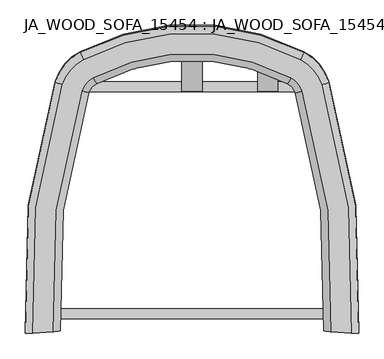
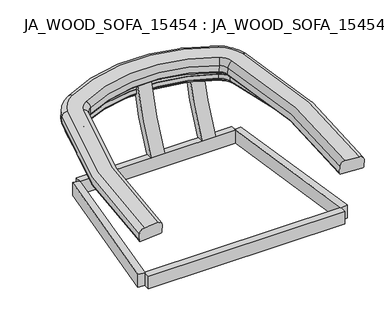
"""IFC4 building model written with IfcOpenShell, lengths in millimetres: furniture geometry, JA_WOOD_SOFA_15454 : JA_WOOD_SOFA_15454."""

from ifc_helpers import new_model, si_unit, point, frame, frame_2d, origin, place, context, project, spatial, polyline, circle_curve, ellipse_curve, trimmed, segment, composite_curve, outline, extrude, source, transform, mapped, element, save
from ifc_brep_helpers import plane_surface, cylinder_surface, revolved_surface, advanced_brep


def ja_wood_sofa_15454_ja_wood_sofa_15454_f522b914(model_context):
    return source(origin(), model_context, "Body", "SolidModel", [
        advanced_brep(
        [(-275.4813305, -35.2597244, 497.0679673), (-315.380229, -38.0910735, 496.8202564), (-330.3423159, -37.8454933, 481.7844443), (-330.3423159, -36.1023784, 461.8605503), (-325.3549536, -35.3126811, 456.9105407), (-265.5066059, -31.0656574, 457.2821072), (-260.5192436, -31.1475174, 462.2940445), (-260.5192436, -32.8906323, 482.2179385), (-256.5569192, 453.6794856, 539.8446054), (-218.4430808, 441.5874987, 538.7866936), (-196.0745351, 468.1438524, 541.1100735), (196.0745351, 468.1438524, 541.1100735), (218.4430808, 441.5874987, 538.7866936), (275.4813305, -35.2597244, 497.0679673), (315.380229, -38.0910735, 496.8202564), (256.5569192, 453.6794856, 539.8446054), (214.6467039, 503.4360732, 544.1977427), (-214.6467039, 503.4360732, 544.1977427), (-270.8496086, 461.2644317, 505.3745079), (-270.8496086, 459.5213169, 525.2984018), (-208.9146212, 442.0507317, 498.6744277), (-266.0853788, 460.1887121, 500.2612954), (-219.2897461, 515.7453581, 505.1218721), (219.2897461, 515.7453581, 505.1218721), (266.0853788, 460.1887121, 500.2612954), (325.3549536, -35.3126811, 456.9105407), (265.5066059, -31.0656574, 457.2821072), (208.9146212, 442.0507317, 498.6744277), (191.4314929, 462.8070269, 500.4903683), (-191.4314929, 462.8070269, 500.4903683), (-204.1503914, 438.3603397, 523.4470562), (-204.1503914, 440.1034546, 503.5231622), (-221.6112672, 519.7211069, 510.4888042), (-221.6112672, 517.9779921, 530.4126982), (-189.1099718, 456.2166058, 525.0092771), (-189.1099718, 457.9597206, 505.0853831), (221.6112672, 519.7211069, 510.4888042), (221.6112672, 517.9779921, 530.4126982), (189.1099718, 456.2166058, 525.0092771), (189.1099718, 457.9597206, 505.0853831), (270.8496086, 461.2644317, 505.3745079), (270.8496086, 459.5213169, 525.2984018), (204.1503914, 438.3603397, 523.4470562), (204.1503914, 440.1034546, 503.5231622), (260.5192436, -32.8906323, 482.2179385), (260.5192436, -31.1475174, 462.2940445), (330.3423159, -36.1023784, 461.8605503), (330.3423159, -37.8454933, 481.7844443)],
        [
            (0, 1),
            (1, 2, circle_curve(frame((-315.380229, -36.7837374, 481.8773359), z_axis=(0.07105411082948589, -0.9936767785792983, -0.08693545333464162), x_axis=(-0.9974724624440673, -0.07078372848595715, -0.006192773804617793)), 15.0)),
            (2, 3),
            (3, 4, circle_curve(frame((-325.3549536, -35.7484598, 461.8915142), z_axis=(0.07105411082948589, -0.9936767785792983, -0.08693545333464162), x_axis=(-0.9974724624440673, -0.07078372848595715, -0.006192773804617793)), 5.0)),
            (4, 5),
            (5, 6, circle_curve(frame((-265.5066059, -31.5014361, 462.2630806), z_axis=(0.07105411082948589, -0.9936767785792983, -0.08693545333464162), x_axis=(-0.9974724624440673, -0.07078372848595715, -0.006192773804617793)), 5.0)),
            (6, 7),
            (7, 0, circle_curve(frame((-275.4813305, -33.9523882, 482.1250469), z_axis=(0.07105411082948589, -0.9936767785792983, -0.08693545333464162), x_axis=(-0.9974724624440673, -0.07078372848595715, -0.006192773804617793)), 15.0)),
            (8, 1, circle_curve(frame((999.4131606, 55.2107286, 504.9831064), z_axis=(0.0, -0.08715574274765152, 0.9961946980917462), x_axis=(-0.9974724624440673, -0.07078372848595717, -0.006192773804617792)), 1318.125)),
            (0, 9, circle_curve(frame((999.4131606, 55.2107286, 504.9831064), z_axis=(0.0, 0.08715574274765152, -0.9961946980917462), x_axis=(-0.9974724624440673, -0.07078372848595717, -0.006192773804617792)), 1278.125)),
            (9, 10, circle_curve(frame((-174.8157372, 427.7462984, 537.5757455), z_axis=(0.0, 0.08715574274765152, -0.9961946980917462), x_axis=(-0.9528459590255555, 0.3022996734028965, 0.026447794410340692)), 45.7863553)),
            (10, 11, circle_curve(frame((0.0, 95.5483916, 508.5121946), z_axis=(0.0, 0.08715574274765152, -0.9961946980917462), x_axis=(-0.4643042190951026, 0.8823055189929315, 0.0771917306782324)), 422.2975521)),
            (11, 12, circle_curve(frame((174.8157372, 427.7462984, 537.5757455), z_axis=(0.0, 0.08715574274765152, -0.9961946980917462), x_axis=(0.46430421909505437, 0.8823055189929567, 0.0771917306782346)), 45.7863553)),
            (12, 13, circle_curve(frame((-999.4131606, 55.2107286, 504.9831064), z_axis=(0.0, 0.08715574274765152, -0.9961946980917462), x_axis=(0.9528459590255144, 0.3022996734030248, 0.026447794410351923)), 1278.125)),
            (13, 14),
            (14, 15, circle_curve(frame((-999.4131606, 55.2107286, 504.9831064), z_axis=(0.0, -0.08715574274765152, 0.9961946980917462), x_axis=(0.9528459590255144, 0.3022996734030248, 0.026447794410351923)), 1318.125)),
            (15, 16, circle_curve(frame((174.8157372, 427.7462984, 537.5757455), z_axis=(0.0, -0.08715574274765152, 0.9961946980917462), x_axis=(0.46430421909505437, 0.8823055189929567, 0.0771917306782346)), 85.7863553)),
            (16, 17, circle_curve(frame((0.0, 95.5483916, 508.5121946), z_axis=(0.0, -0.08715574274765152, 0.9961946980917462), x_axis=(-0.4643042190951026, 0.8823055189929315, 0.0771917306782324)), 462.2975521)),
            (17, 8, circle_curve(frame((-174.8157372, 427.7462984, 537.5757455), z_axis=(0.0, -0.08715574274765152, 0.9961946980917462), x_axis=(-0.9528459590255555, 0.3022996734028965, 0.026447794410340692)), 85.7863553)),
            (18, 3, circle_curve(frame((999.4131606, 58.2611796, 470.1162919), z_axis=(0.0, -0.08715574274765152, 0.9961946980917462), x_axis=(-0.9974724624440673, -0.07078372848595717, -0.006192773804617792)), 1333.125)),
            (2, 19, circle_curve(frame((999.4131606, 56.5180648, 490.0401859), z_axis=(0.0, 0.08715574274765152, -0.9961946980917462), x_axis=(-0.9974724624440673, -0.07078372848595717, -0.006192773804617792)), 1333.125)),
            (19, 18),
            (20, 5, circle_curve(frame((999.4131606, 58.6969583, 465.1353184), z_axis=(0.0, -0.08715574274765152, 0.9961946980917462), x_axis=(-0.9974724624440673, -0.07078372848595717, -0.006192773804617792)), 1268.125)),
            (4, 21, circle_curve(frame((999.4131606, 58.6969583, 465.1353184), z_axis=(0.0, 0.08715574274765152, -0.9961946980917462), x_axis=(-0.9974724624440673, -0.07078372848595717, -0.006192773804617792)), 1328.125)),
            (21, 22, circle_curve(frame((-174.8157372, 431.2325281, 497.7279576), z_axis=(0.0, 0.08715574274765152, -0.9961946980917462), x_axis=(-0.9528459590255555, 0.3022996734028965, 0.026447794410340692)), 95.7863553)),
            (22, 23, circle_curve(frame((0.0, 99.0346213, 468.6644067), z_axis=(0.0, 0.08715574274765152, -0.9961946980917462), x_axis=(-0.4643042190951026, 0.8823055189929315, 0.0771917306782324)), 472.2975521)),
            (23, 24, circle_curve(frame((174.8157372, 431.2325281, 497.7279576), z_axis=(0.0, 0.08715574274765152, -0.9961946980917462), x_axis=(0.46430421909505437, 0.8823055189929567, 0.0771917306782346)), 95.7863553)),
            (24, 25, circle_curve(frame((-999.4131606, 58.6969583, 465.1353184), z_axis=(0.0, 0.08715574274765152, -0.9961946980917462), x_axis=(0.9528459590255144, 0.3022996734030248, 0.026447794410351923)), 1328.125)),
            (25, 26),
            (26, 27, circle_curve(frame((-999.4131606, 58.6969583, 465.1353184), z_axis=(0.0, -0.08715574274765152, 0.9961946980917462), x_axis=(0.9528459590255144, 0.3022996734030248, 0.026447794410351923)), 1268.125)),
            (27, 28, circle_curve(frame((174.8157372, 431.2325281, 497.7279576), z_axis=(0.0, -0.08715574274765152, 0.9961946980917462), x_axis=(0.46430421909505437, 0.8823055189929567, 0.0771917306782346)), 35.7863553)),
            (28, 29, circle_curve(frame((0.0, 99.0346213, 468.6644067), z_axis=(0.0, -0.08715574274765152, 0.9961946980917462), x_axis=(-0.4643042190951026, 0.8823055189929315, 0.0771917306782324)), 412.2975521)),
            (29, 20, circle_curve(frame((-174.8157372, 431.2325281, 497.7279576), z_axis=(0.0, -0.08715574274765152, 0.9961946980917462), x_axis=(-0.9528459590255555, 0.3022996734028965, 0.026447794410340692)), 35.7863553)),
            (30, 7, circle_curve(frame((999.4131606, 56.5180648, 490.0401859), z_axis=(0.0, -0.08715574274765152, 0.9961946980917462), x_axis=(-0.9974724624440673, -0.07078372848595717, -0.006192773804617792)), 1263.125)),
            (6, 31, circle_curve(frame((999.4131606, 58.2611796, 470.1162919), z_axis=(0.0, 0.08715574274765152, -0.9961946980917462), x_axis=(-0.9974724624440673, -0.07078372848595717, -0.006192773804617792)), 1263.125)),
            (31, 30),
            (32, 18, circle_curve(frame((-174.8157372, 430.7967494, 502.708931), z_axis=(0.0, -0.08715574274765152, 0.9961946980917462), x_axis=(-0.9528459590255555, 0.3022996734028965, 0.026447794410340692)), 100.7863553)),
            (19, 33, circle_curve(frame((-174.8157372, 429.0536346, 522.632825), z_axis=(0.0, 0.08715574274765152, -0.9961946980917462), x_axis=(-0.9528459590255555, 0.3022996734028965, 0.026447794410340692)), 100.7863553)),
            (33, 32),
            (34, 30, circle_curve(frame((-174.8157372, 429.0536346, 522.632825), z_axis=(0.0, -0.08715574274765152, 0.9961946980917462), x_axis=(-0.9528459590255555, 0.3022996734028965, 0.026447794410340692)), 30.7863553)),
            (31, 35, circle_curve(frame((-174.8157372, 430.7967494, 502.708931), z_axis=(0.0, 0.08715574274765152, -0.9961946980917462), x_axis=(-0.9528459590255555, 0.3022996734028965, 0.026447794410340692)), 30.7863553)),
            (35, 34),
            (36, 32, circle_curve(frame((0.0, 98.5988426, 473.6453801), z_axis=(0.0, -0.08715574274765152, 0.9961946980917462), x_axis=(-0.4643042190951026, 0.8823055189929315, 0.0771917306782324)), 477.2975521)),
            (33, 37, circle_curve(frame((0.0, 96.8557277, 493.5692741), z_axis=(0.0, 0.08715574274765152, -0.9961946980917462), x_axis=(-0.4643042190951026, 0.8823055189929315, 0.0771917306782324)), 477.2975521)),
            (37, 36),
            (38, 34, circle_curve(frame((0.0, 96.8557277, 493.5692741), z_axis=(0.0, -0.08715574274765152, 0.9961946980917462), x_axis=(-0.4643042190951026, 0.8823055189929315, 0.0771917306782324)), 407.2975521)),
            (35, 39, circle_curve(frame((0.0, 98.5988426, 473.6453801), z_axis=(0.0, 0.08715574274765152, -0.9961946980917462), x_axis=(-0.4643042190951026, 0.8823055189929315, 0.0771917306782324)), 407.2975521)),
            (39, 38),
            (40, 36, circle_curve(frame((174.8157372, 430.7967494, 502.708931), z_axis=(0.0, -0.08715574274765152, 0.9961946980917462), x_axis=(0.46430421909505437, 0.8823055189929567, 0.0771917306782346)), 100.7863553)),
            (37, 41, circle_curve(frame((174.8157372, 429.0536346, 522.632825), z_axis=(0.0, 0.08715574274765152, -0.9961946980917462), x_axis=(0.46430421909505437, 0.8823055189929567, 0.0771917306782346)), 100.7863553)),
            (41, 40),
            (42, 38, circle_curve(frame((174.8157372, 429.0536346, 522.632825), z_axis=(0.0, -0.08715574274765152, 0.9961946980917462), x_axis=(0.46430421909505437, 0.8823055189929567, 0.0771917306782346)), 30.7863553)),
            (39, 43, circle_curve(frame((174.8157372, 430.7967494, 502.708931), z_axis=(0.0, 0.08715574274765152, -0.9961946980917462), x_axis=(0.46430421909505437, 0.8823055189929567, 0.0771917306782346)), 30.7863553)),
            (43, 42),
            (13, 44, circle_curve(frame((275.4813305, -33.9523882, 482.1250469), z_axis=(-0.07105411082947943, -0.9936767785792986, -0.08693545333464163), x_axis=(0.9974724624440677, -0.07078372848595083, -0.006192773804617201)), 15.0)),
            (44, 45),
            (45, 26, circle_curve(frame((265.5066059, -31.5014361, 462.2630806), z_axis=(-0.07105411082947943, -0.9936767785792986, -0.08693545333464163), x_axis=(0.9974724624440677, -0.07078372848595083, -0.006192773804617201)), 5.0)),
            (25, 46, circle_curve(frame((325.3549536, -35.7484598, 461.8915142), z_axis=(-0.07105411082947943, -0.9936767785792986, -0.08693545333464163), x_axis=(0.9974724624440677, -0.07078372848595083, -0.006192773804617201)), 5.0)),
            (46, 47),
            (47, 14, circle_curve(frame((315.380229, -36.7837374, 481.8773359), z_axis=(-0.07105411082947943, -0.9936767785792986, -0.08693545333464163), x_axis=(0.9974724624440677, -0.07078372848595083, -0.006192773804617201)), 15.0)),
            (46, 40, circle_curve(frame((-999.4131606, 58.2611796, 470.1162919), z_axis=(0.0, -0.08715574274765152, 0.9961946980917462), x_axis=(0.9528459590255144, 0.3022996734030248, 0.026447794410351923)), 1333.125)),
            (41, 47, circle_curve(frame((-999.4131606, 56.5180648, 490.0401859), z_axis=(0.0, 0.08715574274765152, -0.9961946980917462), x_axis=(0.9528459590255144, 0.3022996734030248, 0.026447794410351923)), 1333.125)),
            (44, 42, circle_curve(frame((-999.4131606, 56.5180648, 490.0401859), z_axis=(0.0, -0.08715574274765152, 0.9961946980917462), x_axis=(0.9528459590255144, 0.3022996734030248, 0.026447794410351923)), 1263.125)),
            (43, 45, circle_curve(frame((-999.4131606, 58.2611796, 470.1162919), z_axis=(0.0, 0.08715574274765152, -0.9961946980917462), x_axis=(0.9528459590255144, 0.3022996734030248, 0.026447794410351923)), 1263.125)),
            (8, 19, circle_curve(frame((-256.5569192, 454.9868218, 524.9016849), z_axis=(-0.30345440904482285, -0.9492200924793655, -0.08304599728296726), x_axis=(-0.9528459590255172, 0.30229967340301656, 0.026447794410351194)), 15.0)),
            (18, 21, circle_curve(frame((-266.0853788, 459.7529333, 505.2422689), z_axis=(-0.3034544090448216, -0.9492200924793658, -0.0830459972829673), x_axis=(-0.9528459590255175, 0.30229967340301533, 0.026447794410351087)), 5.0)),
            (20, 31, circle_curve(frame((-208.9146212, 441.6149529, 503.6554012), z_axis=(-0.3034544090448277, -0.9492200924793639, -0.08304599728296713), x_axis=(-0.9528459590255156, 0.30229967340302133, 0.026447794410351614)), 5.0)),
            (30, 9, circle_curve(frame((-218.4430808, 442.8948348, 523.8437731), z_axis=(-0.30345440904482823, -0.9492200924793637, -0.08304599728296712), x_axis=(-0.9528459590255154, 0.30229967340302194, 0.026447794410351666)), 15.0)),
            (17, 33, circle_curve(frame((-214.6467039, 504.7434093, 529.2548222), z_axis=(-0.8856757827390686, -0.4625374013641972, -0.040466779076104395), x_axis=(-0.4643042190951301, 0.8823055189929174, 0.07719173067823115)), 15.0)),
            (32, 22, circle_curve(frame((-219.2897461, 515.3095793, 510.1028456), z_axis=(-0.8856757827390704, -0.46253740136419325, -0.04046677907610405), x_axis=(-0.4643042190951262, 0.8823055189929193, 0.07719173067823133)), 5.0)),
            (29, 35, circle_curve(frame((-191.4314929, 462.3712482, 505.4713417), z_axis=(-0.8856757827390473, -0.46253740136423716, -0.04046677907610789), x_axis=(-0.4643042190951703, 0.8823055189928962, 0.0771917306782293)), 5.0)),
            (34, 10, circle_curve(frame((-196.0745351, 469.4511885, 526.167153), z_axis=(-0.8856757827390422, -0.4625374013642469, -0.040466779076108746), x_axis=(-0.46430421909518, 0.8823055189928912, 0.07719173067822886)), 15.0)),
            (16, 37, circle_curve(frame((214.6467039, 504.7434093, 529.2548222), z_axis=(-0.8856757827390904, 0.46253740136415533, 0.040466779076100766), x_axis=(0.4643042190950882, 0.8823055189929391, 0.07719173067823308)), 15.0)),
            (36, 23, circle_curve(frame((219.2897461, 515.3095793, 510.1028456), z_axis=(-0.885675782739091, 0.4625374013641542, 0.04046677907610067), x_axis=(0.46430421909508707, 0.8823055189929396, 0.07719173067823312)), 5.0)),
            (28, 39, circle_curve(frame((191.4314929, 462.3712482, 505.4713417), z_axis=(-0.8856757827390884, 0.46253740136415916, 0.04046677907610111), x_axis=(0.4643042190950921, 0.882305518992937, 0.07719173067823289)), 5.0)),
            (38, 11, circle_curve(frame((196.0745351, 469.4511885, 526.167153), z_axis=(-0.885675782739088, 0.46253740136415983, 0.04046677907610116), x_axis=(0.46430421909509273, 0.8823055189929367, 0.07719173067823286)), 15.0)),
            (15, 41, circle_curve(frame((256.5569192, 454.9868218, 524.9016849), z_axis=(-0.3034544090448294, 0.9492200924793632, 0.08304599728296706), x_axis=(0.9528459590255149, 0.302299673403023, 0.026447794410351767)), 15.0)),
            (40, 24, circle_curve(frame((266.0853788, 459.7529333, 505.2422689), z_axis=(-0.3034544090448297, 0.9492200924793631, 0.08304599728296706), x_axis=(0.9528459590255149, 0.3022996734030232, 0.026447794410351794)), 5.0)),
            (27, 43, circle_curve(frame((208.9146212, 441.6149529, 503.6554012), z_axis=(-0.3034544090448273, 0.9492200924793639, 0.08304599728296713), x_axis=(0.9528459590255158, 0.3022996734030208, 0.02644779441035158)), 5.0)),
            (42, 12, circle_curve(frame((218.4430808, 442.8948348, 523.8437731), z_axis=(-0.30345440904482646, 0.9492200924793643, 0.08304599728296715), x_axis=(0.952845959025516, 0.3022996734030201, 0.026447794410351517)), 15.0)),
        ],
        [
            plane_surface(frame((-295.4307798, -36.6753989, 496.9441119), z_axis=(0.07105411082948591, -0.9936767785792983, -0.08693545333464162), x_axis=(0.0, -0.08715574274765152, 0.9961946980917462))),
            plane_surface(frame((999.4131606, 55.2107286, 504.9831064), z_axis=(0.0, -0.08715574274765152, 0.9961946980917463), x_axis=(-0.9974724624440673, -0.07078372848595717, -0.006192773804617792))),
            cylinder_surface(frame((999.4131606, 55.2107286, 504.9831064), z_axis=(0.0, 0.08715574274765152, -0.9961946980917462), x_axis=(-0.9974724624440673, -0.07078372848595717, -0.006192773804617792)), 1333.125),
            plane_surface(frame((999.4131606, 58.6969583, 465.1353184), z_axis=(0.0, 0.08715574274765152, -0.9961946980917463), x_axis=(-0.9974724624440673, -0.07078372848595717, -0.006192773804617792))),
            revolved_surface(polyline([(-260.51924352466256, -31.147517440314132, 462.2940444709035), (-260.51924352466256, -32.890632301143036, 482.2179384999)]), (999.4131606, 55.2107286, 504.9831064), (0.0, 0.08715574274765152, -0.9961946980917462)),
            cylinder_surface(frame((-174.8157372, 427.7462984, 537.5757455), z_axis=(0.0, 0.08715574274765152, -0.9961946980917462), x_axis=(-0.9528459590255555, 0.3022996734028965, 0.026447794410340692)), 100.7863553),
            revolved_surface(polyline([(-204.15039144073, 440.10345455445133, 503.5231621957927), (-204.15039144073, 438.36033969205954, 523.447056242653)]), (-174.8157372, 427.7462984, 537.5757455), (0.0, 0.08715574274765152, -0.9961946980917462)),
            cylinder_surface(frame((0.0, 95.5483916, 508.5121946), z_axis=(0.0, 0.08715574274765152, -0.9961946980917462), x_axis=(-0.4643042190951026, 0.8823055189929315, 0.0771917306782324)), 477.2975521),
            revolved_surface(polyline([(-189.10997186713738, 457.95972069213684, 505.08538304778114), (-189.10997186713738, 456.2166058290539, 525.0092771025418)]), (0.0, 95.5483916, 508.5121946), (0.0, 0.08715574274765152, -0.9961946980917462)),
            cylinder_surface(frame((174.8157372, 427.7462984, 537.5757455), z_axis=(0.0, 0.08715574274765152, -0.9961946980917462), x_axis=(0.46430421909505437, 0.8823055189929567, 0.0771917306782346)), 100.7863553),
            revolved_surface(polyline([(189.10997185634938, 457.95972059286385, 505.08538304705667), (189.10997185634938, 456.21660573047205, 525.009277093917)]), (174.8157372, 427.7462984, 537.5757455), (0.0, 0.08715574274765152, -0.9961946980917462)),
            plane_surface(frame((295.4307798, -36.6753989, 496.9441119), z_axis=(-0.07105411082947907, -0.9936767785792987, -0.08693545333464163), x_axis=(0.0, -0.08715574274765149, 0.9961946980917462))),
            cylinder_surface(frame((-999.4131606, 55.2107286, 504.9831064), z_axis=(0.0, 0.08715574274765152, -0.9961946980917462), x_axis=(0.9528459590255144, 0.3022996734030248, 0.026447794410351923)), 1333.125),
            revolved_surface(polyline([(204.15039139410294, 440.1034545707062, 503.52316219743716), (204.15039139410294, 438.36033970987734, 523.4470562264337)]), (-999.4131606, 55.2107286, 504.9831064), (0.0, 0.08715574274765152, -0.9961946980917462)),
            revolved_surface(trimmed(ellipse_curve(frame((-315.380229, -36.7837374, 481.8773359), z_axis=(0.07105411082948589, -0.9936767785792983, -0.08693545333464162), x_axis=(-0.9974724624440673, -0.07078372848595715, -0.006192773804617793)), 15.0, 15.0), [point((-315.380229, -38.0910735, 496.8202564))], [point((-330.3423159, -37.8454933, 481.7844443))], True, "CARTESIAN"), (999.4131606, 55.2107286, 504.9831064), (0.0, 0.08715574274765152, -0.9961946980917462)),
            revolved_surface(trimmed(ellipse_curve(frame((-325.3549536, -35.7484598, 461.8915142), z_axis=(0.07105411082948589, -0.9936767785792983, -0.08693545333464162), x_axis=(-0.9974724624440673, -0.07078372848595715, -0.006192773804617793)), 5.0, 5.0), [point((-330.3423159, -36.1023784, 461.8605503))], [point((-325.3549536, -35.3126811, 456.9105407))], True, "CARTESIAN"), (999.4131606, 55.2107286, 504.9831064), (0.0, 0.08715574274765152, -0.9961946980917462)),
            revolved_surface(trimmed(ellipse_curve(frame((-265.5066059, -31.5014361, 462.2630806), z_axis=(0.07105411082948589, -0.9936767785792983, -0.08693545333464162), x_axis=(-0.9974724624440673, -0.07078372848595715, -0.006192773804617793)), 5.0, 5.0), [point((-265.5066059, -31.0656574, 457.2821072))], [point((-260.5192436, -31.1475174, 462.2940445))], True, "CARTESIAN"), (999.4131606, 55.2107286, 504.9831064), (0.0, 0.08715574274765152, -0.9961946980917462)),
            revolved_surface(trimmed(ellipse_curve(frame((-275.4813305, -33.9523882, 482.1250469), z_axis=(0.07105411082948589, -0.9936767785792983, -0.08693545333464162), x_axis=(-0.9974724624440673, -0.07078372848595715, -0.006192773804617793)), 15.0, 15.0), [point((-260.5192436, -32.8906323, 482.2179385))], [point((-275.4813305, -35.2597244, 497.0679673))], True, "CARTESIAN"), (999.4131606, 55.2107286, 504.9831064), (0.0, 0.08715574274765152, -0.9961946980917462)),
            revolved_surface(trimmed(ellipse_curve(frame((-256.5569192, 454.9868218, 524.9016849), z_axis=(-0.3034544090447023, -0.9492200924794036, -0.08304599728297062), x_axis=(-0.9528459590255555, 0.3022996734028964, 0.026447794410340682)), 15.0, 15.0), [point((-256.5569192, 453.6794856, 539.8446054))], [point((-270.8496086, 459.5213169, 525.2984018))], True, "CARTESIAN"), (-174.8157372, 427.7462984, 537.5757455), (0.0, 0.08715574274765152, -0.9961946980917462)),
            revolved_surface(trimmed(ellipse_curve(frame((-266.0853788, 459.7529333, 505.2422689), z_axis=(-0.3034544090447023, -0.9492200924794036, -0.08304599728297062), x_axis=(-0.9528459590255555, 0.3022996734028964, 0.026447794410340682)), 5.0, 5.0), [point((-270.8496086, 461.2644317, 505.3745079))], [point((-266.0853788, 460.1887121, 500.2612954))], True, "CARTESIAN"), (-174.8157372, 427.7462984, 537.5757455), (0.0, 0.08715574274765152, -0.9961946980917462)),
            revolved_surface(trimmed(ellipse_curve(frame((-208.9146212, 441.6149529, 503.6554012), z_axis=(-0.3034544090447023, -0.9492200924794036, -0.08304599728297062), x_axis=(-0.9528459590255555, 0.3022996734028964, 0.026447794410340682)), 5.0, 5.0), [point((-208.9146212, 442.0507317, 498.6744277))], [point((-204.1503914, 440.1034546, 503.5231622))], True, "CARTESIAN"), (-174.8157372, 427.7462984, 537.5757455), (0.0, 0.08715574274765152, -0.9961946980917462)),
            revolved_surface(trimmed(ellipse_curve(frame((-218.4430808, 442.8948348, 523.8437731), z_axis=(-0.3034544090447023, -0.9492200924794036, -0.08304599728297062), x_axis=(-0.9528459590255555, 0.3022996734028964, 0.026447794410340682)), 15.0, 15.0), [point((-204.1503914, 438.3603397, 523.4470562))], [point((-218.4430808, 441.5874987, 538.7866936))], True, "CARTESIAN"), (-174.8157372, 427.7462984, 537.5757455), (0.0, 0.08715574274765152, -0.9961946980917462)),
            revolved_surface(trimmed(ellipse_curve(frame((-214.6467039, 504.7434093, 529.2548222), z_axis=(-0.8856757827390829, -0.4625374013641697, -0.04046677907610196), x_axis=(-0.4643042190951026, 0.8823055189929315, 0.07719173067823241)), 15.0, 15.0), [point((-214.6467039, 503.4360732, 544.1977427))], [point((-221.6112672, 517.9779921, 530.4126982))], True, "CARTESIAN"), (0.0, 95.5483916, 508.5121946), (0.0, 0.08715574274765152, -0.9961946980917462)),
            revolved_surface(trimmed(ellipse_curve(frame((-219.2897461, 515.3095793, 510.1028456), z_axis=(-0.8856757827390829, -0.4625374013641697, -0.04046677907610196), x_axis=(-0.4643042190951026, 0.8823055189929315, 0.07719173067823241)), 5.0, 5.0), [point((-221.6112672, 519.7211069, 510.4888042))], [point((-219.2897461, 515.7453581, 505.1218721))], True, "CARTESIAN"), (0.0, 95.5483916, 508.5121946), (0.0, 0.08715574274765152, -0.9961946980917462)),
            revolved_surface(trimmed(ellipse_curve(frame((-191.4314929, 462.3712482, 505.4713417), z_axis=(-0.8856757827390829, -0.4625374013641697, -0.04046677907610196), x_axis=(-0.4643042190951026, 0.8823055189929315, 0.07719173067823241)), 5.0, 5.0), [point((-191.4314929, 462.8070269, 500.4903683))], [point((-189.1099718, 457.9597206, 505.0853831))], True, "CARTESIAN"), (0.0, 95.5483916, 508.5121946), (0.0, 0.08715574274765152, -0.9961946980917462)),
            revolved_surface(trimmed(ellipse_curve(frame((-196.0745351, 469.4511885, 526.167153), z_axis=(-0.8856757827390829, -0.4625374013641697, -0.04046677907610196), x_axis=(-0.4643042190951026, 0.8823055189929315, 0.07719173067823241)), 15.0, 15.0), [point((-189.1099718, 456.2166058, 525.0092771))], [point((-196.0745351, 468.1438524, 541.1100735))], True, "CARTESIAN"), (0.0, 95.5483916, 508.5121946), (0.0, 0.08715574274765152, -0.9961946980917462)),
            revolved_surface(trimmed(ellipse_curve(frame((214.6467039, 504.7434093, 529.2548222), z_axis=(-0.8856757827391082, 0.46253740136412164, 0.04046677907609777), x_axis=(0.4643042190950543, 0.8823055189929567, 0.07719173067823461)), 15.0, 15.0), [point((214.6467039, 503.4360732, 544.1977427))], [point((221.6112672, 517.9779921, 530.4126982))], True, "CARTESIAN"), (174.8157372, 427.7462984, 537.5757455), (0.0, 0.08715574274765152, -0.9961946980917462)),
            revolved_surface(trimmed(ellipse_curve(frame((219.2897461, 515.3095793, 510.1028456), z_axis=(-0.8856757827391082, 0.46253740136412164, 0.04046677907609777), x_axis=(0.4643042190950543, 0.8823055189929567, 0.07719173067823461)), 5.0, 5.0), [point((221.6112672, 519.7211069, 510.4888042))], [point((219.2897461, 515.7453581, 505.1218721))], True, "CARTESIAN"), (174.8157372, 427.7462984, 537.5757455), (0.0, 0.08715574274765152, -0.9961946980917462)),
            revolved_surface(trimmed(ellipse_curve(frame((191.4314929, 462.3712482, 505.4713417), z_axis=(-0.8856757827391082, 0.46253740136412164, 0.04046677907609777), x_axis=(0.4643042190950543, 0.8823055189929567, 0.07719173067823461)), 5.0, 5.0), [point((191.4314929, 462.8070269, 500.4903683))], [point((189.1099718, 457.9597206, 505.0853831))], True, "CARTESIAN"), (174.8157372, 427.7462984, 537.5757455), (0.0, 0.08715574274765152, -0.9961946980917462)),
            revolved_surface(trimmed(ellipse_curve(frame((196.0745351, 469.4511885, 526.167153), z_axis=(-0.8856757827391082, 0.46253740136412164, 0.04046677907609777), x_axis=(0.4643042190950543, 0.8823055189929567, 0.07719173067823461)), 15.0, 15.0), [point((189.1099718, 456.2166058, 525.0092771))], [point((196.0745351, 468.1438524, 541.1100735))], True, "CARTESIAN"), (174.8157372, 427.7462984, 537.5757455), (0.0, 0.08715574274765152, -0.9961946980917462)),
            revolved_surface(trimmed(ellipse_curve(frame((256.5569192, 454.9868218, 524.9016849), z_axis=(-0.3034544090448312, 0.9492200924793627, 0.08304599728296702), x_axis=(0.9528459590255144, 0.30229967340302477, 0.026447794410351954)), 15.0, 15.0), [point((256.5569192, 453.6794856, 539.8446054))], [point((270.8496086, 459.5213169, 525.2984018))], True, "CARTESIAN"), (-999.4131606, 55.2107286, 504.9831064), (0.0, 0.08715574274765152, -0.9961946980917462)),
            revolved_surface(trimmed(ellipse_curve(frame((266.0853788, 459.7529333, 505.2422689), z_axis=(-0.3034544090448312, 0.9492200924793627, 0.08304599728296702), x_axis=(0.9528459590255144, 0.30229967340302477, 0.026447794410351954)), 5.0, 5.0), [point((270.8496086, 461.2644317, 505.3745079))], [point((266.0853788, 460.1887121, 500.2612954))], True, "CARTESIAN"), (-999.4131606, 55.2107286, 504.9831064), (0.0, 0.08715574274765152, -0.9961946980917462)),
            revolved_surface(trimmed(ellipse_curve(frame((208.9146212, 441.6149529, 503.6554012), z_axis=(-0.3034544090448312, 0.9492200924793627, 0.08304599728296702), x_axis=(0.9528459590255144, 0.30229967340302477, 0.026447794410351954)), 5.0, 5.0), [point((208.9146212, 442.0507317, 498.6744277))], [point((204.1503914, 440.1034546, 503.5231622))], True, "CARTESIAN"), (-999.4131606, 55.2107286, 504.9831064), (0.0, 0.08715574274765152, -0.9961946980917462)),
            revolved_surface(trimmed(ellipse_curve(frame((218.4430808, 442.8948348, 523.8437731), z_axis=(-0.3034544090448312, 0.9492200924793627, 0.08304599728296702), x_axis=(0.9528459590255144, 0.30229967340302477, 0.026447794410351954)), 15.0, 15.0), [point((204.1503914, 438.3603397, 523.4470562))], [point((218.4430808, 441.5874987, 538.7866936))], True, "CARTESIAN"), (-999.4131606, 55.2107286, 504.9831064), (0.0, 0.08715574274765152, -0.9961946980917462)),
        ],
        [
            (0, [[1, 2, 3, 4, 5, 6, 7, 8]]),
            (1, [[9, -1, 10, 11, 12, 13, 14, 15, 16, 17, 18, 19]]),
            (2, [[20, -3, 21, 22]]),
            (3, [[23, -5, 24, 25, 26, 27, 28, 29, 30, 31, 32, 33]]),
            (4, [[34, -7, 35, 36]]),
            (5, [[37, -22, 38, 39]]),
            (6, [[40, -36, 41, 42]]),
            (7, [[43, -39, 44, 45]]),
            (8, [[46, -42, 47, 48]]),
            (9, [[49, -45, 50, 51]]),
            (10, [[52, -48, 53, 54]]),
            (11, [[55, 56, 57, -29, 58, 59, 60, -15]]),
            (12, [[61, -51, 62, -59]]),
            (13, [[63, -54, 64, -56]]),
            (14, [[-21, -2, -9, 65]]),
            (15, [[-24, -4, -20, 66]]),
            (16, [[-35, -6, -23, 67]]),
            (17, [[-10, -8, -34, 68]]),
            (18, [[-38, -65, -19, 69]]),
            (19, [[-25, -66, -37, 70]]),
            (20, [[-41, -67, -33, 71]]),
            (21, [[-11, -68, -40, 72]]),
            (22, [[-44, -69, -18, 73]]),
            (23, [[-26, -70, -43, 74]]),
            (24, [[-47, -71, -32, 75]]),
            (25, [[-12, -72, -46, 76]]),
            (26, [[-50, -73, -17, 77]]),
            (27, [[-27, -74, -49, 78]]),
            (28, [[-53, -75, -31, 79]]),
            (29, [[-13, -76, -52, 80]]),
            (30, [[-62, -77, -16, -60]]),
            (31, [[-28, -78, -61, -58]]),
            (32, [[-64, -79, -30, -57]]),
            (33, [[-14, -80, -63, -55]]),
        ],
    ),
        extrude(outline(polyline([(287.6258394, 7.4007211), (227.593365, 443.6367016), (247.406635, 446.3632984), (307.4391094, 10.1273179), (287.6258394, 7.4007211)])), frame((0.0, 0.0, 280.0), z_axis=(0.0, 0.0, 1.0), x_axis=(1.0, 0.0, 0.0)), (0.0, 0.0, 1.0), 40.0),
        extrude(outline(polyline([(-287.6258394, 7.4007211), (-307.4391094, 10.1273179), (-247.406635, 446.3632984), (-227.593365, 443.6367016), (-287.6258394, 7.4007211)])), frame((0.0, 0.0, 280.0), z_axis=(0.0, 0.0, 1.0), x_axis=(1.0, 0.0, 0.0)), (0.0, 0.0, 1.0), 40.0),
        extrude(outline(polyline([(228.5, 460.0), (228.5, 440.0), (-228.5, 440.0), (-228.5, 460.0), (228.5, 460.0)])), frame((0.0, 0.0, 280.0), z_axis=(0.0, 0.0, 1.0), x_axis=(1.0, 0.0, 0.0)), (0.0, 0.0, 1.0), 40.0),
        advanced_brep(
        [(-273.0114083, 15.8209103, 490.0), (-322.9838999, 14.1625745, 490.0), (-322.9838999, 14.1625745, 477.0710678), (-321.5202395, 14.2111461, 473.5355339), (-307.9921524, 14.6600753, 460.0), (-288.0031558, 15.3234096, 460.0), (-274.4750687, 15.7723388, 473.5355339), (-273.0114083, 15.8209103, 477.0710678), (-261.321149, 459.5543995, 490.0), (-213.678851, 444.381679, 490.0), (-193.753014, 468.1283669, 490.0), (193.753014, 468.1283669, 490.0), (213.678851, 444.381679, 490.0), (273.0114083, 15.8209103, 490.0), (322.9838999, 14.1625745, 490.0), (261.321149, 459.5543995, 490.0), (216.968225, 512.412156, 490.0), (-216.968225, 512.412156, 490.0), (-261.321149, 459.5543995, 477.0710678), (-227.9715404, 448.9334952, 460.0), (-247.0284596, 455.0025834, 460.0), (-210.0036617, 499.1270193, 460.0), (210.0036617, 499.1270193, 460.0), (247.0284596, 455.0025834, 460.0), (307.9921524, 14.6600753, 460.0), (288.0031558, 15.3234096, 460.0), (227.9715404, 448.9334952, 460.0), (200.7175773, 481.4135036, 460.0), (-200.7175773, 481.4135036, 460.0), (-213.678851, 444.381679, 477.0710678), (-216.968225, 512.412156, 477.0710678), (-193.753014, 468.1283669, 477.0710678), (216.968225, 512.412156, 477.0710678), (193.753014, 468.1283669, 477.0710678), (261.321149, 459.5543995, 477.0710678), (213.678851, 444.381679, 477.0710678), (273.0114083, 15.8209103, 477.0710678), (274.4750687, 15.7723388, 473.5355339), (321.5202395, 14.2111461, 473.5355339), (322.9838999, 14.1625745, 477.0710678), (-259.9257384, 459.1100008, 473.5355339), (-215.0742616, 444.8260777, 473.5355339), (-216.2882672, 511.1151138, 473.5355339), (-194.4329718, 469.425409, 473.5355339), (216.2882672, 511.1151138, 473.5355339), (194.4329718, 469.425409, 473.5355339), (259.9257384, 459.1100008, 473.5355339), (215.0742616, 444.8260777, 473.5355339)],
        [
            (0, 1),
            (1, 2),
            (2, 3, circle_curve(frame((-317.9866508, 14.3284081, 477.0710678), z_axis=(0.03316671516456435, -0.9994498331608208, 0.0), x_axis=(-0.9994498331608208, -0.03316671516456435, 0.0)), 5.0)),
            (3, 4),
            (4, 5),
            (5, 6),
            (6, 7, circle_curve(frame((-278.0086574, 15.6550767, 477.0710678), z_axis=(0.03316671516456435, -0.9994498331608208, 0.0), x_axis=(-0.9994498331608208, -0.03316671516456435, 0.0)), 5.0)),
            (7, 0),
            (8, 1, circle_curve(frame((999.4131606, 58.0462845, 490.0), z_axis=(0.0, 0.0, 1.0), x_axis=(-0.9994498331608208, -0.03316671516456434, 0.0)), 1323.125)),
            (0, 9, circle_curve(frame((999.4131606, 58.0462845, 490.0), z_axis=(0.0, 0.0, -1.0), x_axis=(-0.9994498331608208, -0.03316671516456434, 0.0)), 1273.125)),
            (9, 10, circle_curve(frame((-174.8157372, 432.0048797, 490.0), z_axis=(0.0, 0.0, -1.0), x_axis=(-0.9528459590255557, 0.3034544090447015, 0.0)), 40.7863553)),
            (10, 11, circle_curve(frame((0.0, 98.5380308, 490.0), z_axis=(0.0, 0.0, -1.0), x_axis=(-0.4643042190951026, 0.8856757827390828, 0.0)), 417.2975521)),
            (11, 12, circle_curve(frame((174.8157372, 432.0048797, 490.0), z_axis=(0.0, 0.0, -1.0), x_axis=(0.4643042190950552, 0.8856757827391076, 0.0)), 40.7863553)),
            (12, 13, circle_curve(frame((-999.4131606, 58.0462845, 490.0), z_axis=(0.0, 0.0, -1.0), x_axis=(0.9528459590255144, 0.3034544090448312, 0.0)), 1273.125)),
            (13, 14),
            (14, 15, circle_curve(frame((-999.4131606, 58.0462845, 490.0), z_axis=(0.0, 0.0, 1.0), x_axis=(0.9528459590255144, 0.3034544090448312, 0.0)), 1323.125)),
            (15, 16, circle_curve(frame((174.8157372, 432.0048797, 490.0), z_axis=(0.0, 0.0, 1.0), x_axis=(0.4643042190950552, 0.8856757827391076, 0.0)), 90.7863553)),
            (16, 17, circle_curve(frame((0.0, 98.5380308, 490.0), z_axis=(0.0, 0.0, 1.0), x_axis=(-0.4643042190951026, 0.8856757827390828, 0.0)), 467.2975521)),
            (17, 8, circle_curve(frame((-174.8157372, 432.0048797, 490.0), z_axis=(0.0, 0.0, 1.0), x_axis=(-0.9528459590255557, 0.3034544090447015, 0.0)), 90.7863553)),
            (18, 2, circle_curve(frame((999.4131606, 58.0462845, 477.0710678), z_axis=(0.0, 0.0, 1.0), x_axis=(-0.9994498331608208, -0.03316671516456434, 0.0)), 1323.125)),
            (8, 18),
            (19, 5, circle_curve(frame((999.4131606, 58.0462845, 460.0), z_axis=(0.0, 0.0, 1.0), x_axis=(-0.9994498331608208, -0.03316671516456434, 0.0)), 1288.125)),
            (4, 20, circle_curve(frame((999.4131606, 58.0462845, 460.0), z_axis=(0.0, 0.0, -1.0), x_axis=(-0.9994498331608208, -0.03316671516456434, 0.0)), 1308.125)),
            (20, 21, circle_curve(frame((-174.8157372, 432.0048797, 460.0), z_axis=(0.0, 0.0, -1.0), x_axis=(-0.9528459590255557, 0.3034544090447015, 0.0)), 75.7863553)),
            (21, 22, circle_curve(frame((0.0, 98.5380308, 460.0), z_axis=(0.0, 0.0, -1.0), x_axis=(-0.4643042190951026, 0.8856757827390828, 0.0)), 452.2975521)),
            (22, 23, circle_curve(frame((174.8157372, 432.0048797, 460.0), z_axis=(0.0, 0.0, -1.0), x_axis=(0.4643042190950552, 0.8856757827391076, 0.0)), 75.7863553)),
            (23, 24, circle_curve(frame((-999.4131606, 58.0462845, 460.0), z_axis=(0.0, 0.0, -1.0), x_axis=(0.9528459590255144, 0.3034544090448312, 0.0)), 1308.125)),
            (24, 25),
            (25, 26, circle_curve(frame((-999.4131606, 58.0462845, 460.0), z_axis=(0.0, 0.0, 1.0), x_axis=(0.9528459590255144, 0.3034544090448312, 0.0)), 1288.125)),
            (26, 27, circle_curve(frame((174.8157372, 432.0048797, 460.0), z_axis=(0.0, 0.0, 1.0), x_axis=(0.4643042190950552, 0.8856757827391076, 0.0)), 55.7863553)),
            (27, 28, circle_curve(frame((0.0, 98.5380308, 460.0), z_axis=(0.0, 0.0, 1.0), x_axis=(-0.4643042190951026, 0.8856757827390828, 0.0)), 432.2975521)),
            (28, 19, circle_curve(frame((-174.8157372, 432.0048797, 460.0), z_axis=(0.0, 0.0, 1.0), x_axis=(-0.9528459590255557, 0.3034544090447015, 0.0)), 55.7863553)),
            (7, 29, circle_curve(frame((999.4131606, 58.0462845, 477.0710678), z_axis=(0.0, 0.0, -1.0), x_axis=(-0.9994498331608208, -0.03316671516456434, 0.0)), 1273.125)),
            (29, 9),
            (30, 18, circle_curve(frame((-174.8157372, 432.0048797, 477.0710678), z_axis=(0.0, 0.0, 1.0), x_axis=(-0.9528459590255557, 0.3034544090447015, 0.0)), 90.7863553)),
            (17, 30),
            (29, 31, circle_curve(frame((-174.8157372, 432.0048797, 477.0710678), z_axis=(0.0, 0.0, -1.0), x_axis=(-0.9528459590255557, 0.3034544090447015, 0.0)), 40.7863553)),
            (31, 10),
            (32, 30, circle_curve(frame((0.0, 98.5380308, 477.0710678), z_axis=(0.0, 0.0, 1.0), x_axis=(-0.4643042190951026, 0.8856757827390828, 0.0)), 467.2975521)),
            (16, 32),
            (31, 33, circle_curve(frame((0.0, 98.5380308, 477.0710678), z_axis=(0.0, 0.0, -1.0), x_axis=(-0.4643042190951026, 0.8856757827390828, 0.0)), 417.2975521)),
            (33, 11),
            (34, 32, circle_curve(frame((174.8157372, 432.0048797, 477.0710678), z_axis=(0.0, 0.0, 1.0), x_axis=(0.4643042190950552, 0.8856757827391076, 0.0)), 90.7863553)),
            (15, 34),
            (33, 35, circle_curve(frame((174.8157372, 432.0048797, 477.0710678), z_axis=(0.0, 0.0, -1.0), x_axis=(0.4643042190950552, 0.8856757827391076, 0.0)), 40.7863553)),
            (35, 12),
            (13, 36),
            (36, 37, circle_curve(frame((278.0086574, 15.6550767, 477.0710678), z_axis=(-0.033166715164558824, -0.999449833160821, 0.0), x_axis=(0.999449833160821, -0.033166715164558824, 0.0)), 5.0)),
            (37, 25),
            (24, 38),
            (38, 39, circle_curve(frame((317.9866508, 14.3284081, 477.0710678), z_axis=(-0.033166715164558824, -0.999449833160821, 0.0), x_axis=(0.999449833160821, -0.033166715164558824, 0.0)), 5.0)),
            (39, 14),
            (39, 34, circle_curve(frame((-999.4131606, 58.0462845, 477.0710678), z_axis=(0.0, 0.0, 1.0), x_axis=(0.9528459590255144, 0.3034544090448312, 0.0)), 1323.125)),
            (35, 36, circle_curve(frame((-999.4131606, 58.0462845, 477.0710678), z_axis=(0.0, 0.0, -1.0), x_axis=(0.9528459590255144, 0.3034544090448312, 0.0)), 1273.125)),
            (40, 3, circle_curve(frame((999.4131606, 58.0462845, 473.5355339), z_axis=(0.0, 0.0, 1.0), x_axis=(-0.9994498331608208, -0.03316671516456434, 0.0)), 1321.6605339)),
            (18, 40, circle_curve(frame((-256.5569192, 458.0371275, 477.0710678), z_axis=(-0.3034544090448225, -0.9528459590255172, 0.0), x_axis=(-0.9528459590255172, 0.3034544090448225, 0.0)), 5.0)),
            (40, 20),
            (41, 6, circle_curve(frame((999.4131606, 58.0462845, 473.5355339), z_axis=(0.0, 0.0, 1.0), x_axis=(-0.9994498331608208, -0.03316671516456434, 0.0)), 1274.5894661)),
            (19, 41),
            (41, 29, circle_curve(frame((-218.4430808, 445.8989511, 477.0710678), z_axis=(-0.30345440904482707, -0.9528459590255157, 0.0), x_axis=(-0.9528459590255157, 0.30345440904482707, 0.0)), 5.0)),
            (42, 40, circle_curve(frame((-174.8157372, 432.0048797, 473.5355339), z_axis=(0.0, 0.0, 1.0), x_axis=(-0.9528459590255557, 0.3034544090447015, 0.0)), 89.3218892)),
            (30, 42, circle_curve(frame((-214.6467039, 507.9837771, 477.0710678), z_axis=(-0.8856757827390687, -0.46430421909512964, 0.0), x_axis=(-0.46430421909512964, 0.8856757827390687, 0.0)), 5.0)),
            (42, 21),
            (43, 41, circle_curve(frame((-174.8157372, 432.0048797, 473.5355339), z_axis=(0.0, 0.0, 1.0), x_axis=(-0.9528459590255557, 0.3034544090447015, 0.0)), 42.2508214)),
            (28, 43),
            (43, 31, circle_curve(frame((-196.0745351, 472.5567458, 477.0710678), z_axis=(-0.8856757827390525, -0.4643042190951604, 0.0), x_axis=(-0.4643042190951604, 0.8856757827390525, 0.0)), 5.0)),
            (44, 42, circle_curve(frame((0.0, 98.5380308, 473.5355339), z_axis=(0.0, 0.0, 1.0), x_axis=(-0.4643042190951026, 0.8856757827390828, 0.0)), 465.833086)),
            (32, 44, circle_curve(frame((214.6467039, 507.9837771, 477.0710678), z_axis=(-0.8856757827390906, 0.46430421909508784, 0.0), x_axis=(0.46430421909508784, 0.8856757827390906, 0.0)), 5.0)),
            (44, 22),
            (45, 43, circle_curve(frame((0.0, 98.5380308, 473.5355339), z_axis=(0.0, 0.0, 1.0), x_axis=(-0.4643042190951026, 0.8856757827390828, 0.0)), 418.7620182)),
            (27, 45),
            (45, 33, circle_curve(frame((196.0745351, 472.5567458, 477.0710678), z_axis=(-0.8856757827390886, 0.46430421909509156, 0.0), x_axis=(0.46430421909509156, 0.8856757827390886, 0.0)), 5.0)),
            (46, 44, circle_curve(frame((174.8157372, 432.0048797, 473.5355339), z_axis=(0.0, 0.0, 1.0), x_axis=(0.4643042190950552, 0.8856757827391076, 0.0)), 89.3218892)),
            (34, 46, circle_curve(frame((256.5569192, 458.0371275, 477.0710678), z_axis=(-0.3034544090448284, 0.9528459590255154, 0.0), x_axis=(0.9528459590255154, 0.3034544090448284, 0.0)), 5.0)),
            (46, 23),
            (47, 45, circle_curve(frame((174.8157372, 432.0048797, 473.5355339), z_axis=(0.0, 0.0, 1.0), x_axis=(0.4643042190950552, 0.8856757827391076, 0.0)), 42.2508214)),
            (26, 47),
            (47, 35, circle_curve(frame((218.4430808, 445.8989511, 477.0710678), z_axis=(-0.30345440904482507, 0.9528459590255163, 0.0), x_axis=(0.9528459590255163, 0.30345440904482507, 0.0)), 5.0)),
            (38, 46, circle_curve(frame((-999.4131606, 58.0462845, 473.5355339), z_axis=(0.0, 0.0, 1.0), x_axis=(0.9528459590255144, 0.3034544090448312, 0.0)), 1321.6605339)),
            (37, 47, circle_curve(frame((-999.4131606, 58.0462845, 473.5355339), z_axis=(0.0, 0.0, 1.0), x_axis=(0.9528459590255144, 0.3034544090448312, 0.0)), 1274.5894661)),
        ],
        [
            plane_surface(frame((-297.9976541, 14.9917424, 490.0), z_axis=(0.033166715164564355, -0.9994498331608209, 0.0), x_axis=(0.0, 0.0, 1.0))),
            plane_surface(frame((999.4131606, 58.0462845, 490.0), z_axis=(0.0, 0.0, 1.0), x_axis=(-0.9994498331608209, -0.03316671516456435, 0.0))),
            cylinder_surface(frame((999.4131606, 58.0462845, 490.0), z_axis=(0.0, 0.0, -1.0), x_axis=(-0.9994498331608208, -0.03316671516456434, 0.0)), 1323.125),
            plane_surface(frame((999.4131606, 58.0462845, 460.0), z_axis=(0.0, 0.0, -1.0), x_axis=(-0.9994498331608209, -0.03316671516456435, 0.0))),
            revolved_surface(polyline([(-273.01140824287006, 15.820910256114026, 477.0710678), (-273.01140824287006, 15.820910256114026, 490.0)]), (999.4131606, 58.0462845, 490.0), (0.0, 0.0, -1.0)),
            cylinder_surface(frame((-174.8157372, 432.0048797, 490.0), z_axis=(0.0, 0.0, -1.0), x_axis=(-0.9528459590255557, 0.3034544090447015, 0.0)), 90.7863553),
            revolved_surface(polyline([(-213.67885103098556, 444.3816790446487, 477.0710678), (-213.67885103098556, 444.3816790446487, 490.0)]), (-174.8157372, 432.0048797, 490.0), (0.0, 0.0, -1.0)),
            cylinder_surface(frame((0.0, 98.5380308, 490.0), z_axis=(0.0, 0.0, -1.0), x_axis=(-0.4643042190951026, 0.8856757827390828, 0.0)), 467.2975521),
            revolved_surface(polyline([(-193.7530140580884, 468.1283668912707, 477.0710678), (-193.7530140580884, 468.1283668912707, 490.0)]), (0.0, 98.5380308, 490.0), (0.0, 0.0, -1.0)),
            cylinder_surface(frame((174.8157372, 432.0048797, 490.0), z_axis=(0.0, 0.0, -1.0), x_axis=(0.4643042190950552, 0.8856757827391076, 0.0)), 90.7863553),
            revolved_surface(polyline([(193.75301404729996, 468.1283668554029, 477.0710678), (193.75301404729996, 468.1283668554029, 490.0)]), (174.8157372, 432.0048797, 490.0), (0.0, 0.0, -1.0)),
            plane_surface(frame((297.9976541, 14.9917424, 490.0), z_axis=(-0.033166715164558595, -0.9994498331608211, 0.0), x_axis=(0.0, 0.0, 1.0))),
            cylinder_surface(frame((-999.4131606, 58.0462845, 490.0), z_axis=(0.0, 0.0, -1.0), x_axis=(0.9528459590255144, 0.3034544090448312, 0.0)), 1323.125),
            revolved_surface(polyline([(213.67885098435806, 444.3816790152007, 477.0710678), (213.67885098435806, 444.3816790152007, 490.0)]), (-999.4131606, 58.0462845, 490.0), (0.0, 0.0, -1.0)),
            revolved_surface(trimmed(ellipse_curve(frame((-317.9866508, 14.3284081, 477.0710678), z_axis=(0.03316671516456435, -0.9994498331608208, 0.0), x_axis=(-0.9994498331608208, -0.03316671516456435, 0.0)), 5.0, 5.0), [point((-322.9838999, 14.1625745, 477.0710678))], [point((-321.5202395, 14.2111461, 473.5355339))], True, "CARTESIAN"), (999.4131606, 58.0462845, 490.0), (0.0, 0.0, -1.0)),
            revolved_surface(polyline([(-321.5202395, 14.2111461, 473.5355339), (-307.9921524, 14.6600753, 460.0)]), (999.4131606, 58.0462845, 490.0), (0.0, 0.0, -1.0)),
            revolved_surface(polyline([(-288.0031558, 15.3234096, 460.0), (-274.4750687, 15.7723388, 473.5355339)]), (999.4131606, 58.0462845, 490.0), (0.0, 0.0, -1.0)),
            revolved_surface(trimmed(ellipse_curve(frame((-278.0086574, 15.6550767, 477.0710678), z_axis=(0.03316671516456435, -0.9994498331608208, 0.0), x_axis=(-0.9994498331608208, -0.03316671516456435, 0.0)), 5.0, 5.0), [point((-274.4750687, 15.7723388, 473.5355339))], [point((-273.0114083, 15.8209103, 477.0710678))], True, "CARTESIAN"), (999.4131606, 58.0462845, 490.0), (0.0, 0.0, -1.0)),
            revolved_surface(trimmed(ellipse_curve(frame((-256.5569192, 458.0371275, 477.0710678), z_axis=(-0.3034544090447015, -0.9528459590255557, 0.0), x_axis=(-0.9528459590255557, 0.3034544090447015, 0.0)), 5.0, 5.0), [point((-261.321149, 459.5543995, 477.0710678))], [point((-259.9257384, 459.1100008, 473.5355339))], True, "CARTESIAN"), (-174.8157372, 432.0048797, 490.0), (0.0, 0.0, -1.0)),
            revolved_surface(polyline([(-259.9257384, 459.1100008, 473.5355339), (-247.0284596, 455.0025834, 460.0)]), (-174.8157372, 432.0048797, 490.0), (0.0, 0.0, -1.0)),
            revolved_surface(polyline([(-227.9715404, 448.9334952, 460.0), (-215.0742616, 444.8260777, 473.5355339)]), (-174.8157372, 432.0048797, 490.0), (0.0, 0.0, -1.0)),
            revolved_surface(trimmed(ellipse_curve(frame((-218.4430808, 445.8989511, 477.0710678), z_axis=(-0.3034544090447015, -0.9528459590255557, 0.0), x_axis=(-0.9528459590255557, 0.3034544090447015, 0.0)), 5.0, 5.0), [point((-215.0742616, 444.8260777, 473.5355339))], [point((-213.678851, 444.381679, 477.0710678))], True, "CARTESIAN"), (-174.8157372, 432.0048797, 490.0), (0.0, 0.0, -1.0)),
            revolved_surface(trimmed(ellipse_curve(frame((-214.6467039, 507.9837771, 477.0710678), z_axis=(-0.8856757827390828, -0.46430421909510255, 0.0), x_axis=(-0.46430421909510255, 0.8856757827390828, 0.0)), 5.0, 5.0), [point((-216.968225, 512.412156, 477.0710678))], [point((-216.2882672, 511.1151138, 473.5355339))], True, "CARTESIAN"), (0.0, 98.5380308, 490.0), (0.0, 0.0, -1.0)),
            revolved_surface(polyline([(-216.2882672, 511.1151138, 473.5355339), (-210.0036617, 499.1270193, 460.0)]), (0.0, 98.5380308, 490.0), (0.0, 0.0, -1.0)),
            revolved_surface(polyline([(-200.7175773, 481.4135036, 460.0), (-194.4329718, 469.425409, 473.5355339)]), (0.0, 98.5380308, 490.0), (0.0, 0.0, -1.0)),
            revolved_surface(trimmed(ellipse_curve(frame((-196.0745351, 472.5567458, 477.0710678), z_axis=(-0.8856757827390828, -0.46430421909510255, 0.0), x_axis=(-0.46430421909510255, 0.8856757827390828, 0.0)), 5.0, 5.0), [point((-194.4329718, 469.425409, 473.5355339))], [point((-193.753014, 468.1283669, 477.0710678))], True, "CARTESIAN"), (0.0, 98.5380308, 490.0), (0.0, 0.0, -1.0)),
            revolved_surface(trimmed(ellipse_curve(frame((214.6467039, 507.9837771, 477.0710678), z_axis=(-0.8856757827391075, 0.4643042190950554, 0.0), x_axis=(0.4643042190950554, 0.8856757827391075, 0.0)), 5.0, 5.0), [point((216.968225, 512.412156, 477.0710678))], [point((216.2882672, 511.1151138, 473.5355339))], True, "CARTESIAN"), (174.8157372, 432.0048797, 490.0), (0.0, 0.0, -1.0)),
            revolved_surface(polyline([(216.2882672, 511.1151138, 473.5355339), (210.0036617, 499.1270193, 460.0)]), (174.8157372, 432.0048797, 490.0), (0.0, 0.0, -1.0)),
            revolved_surface(polyline([(200.7175773, 481.4135036, 460.0), (194.4329718, 469.425409, 473.5355339)]), (174.8157372, 432.0048797, 490.0), (0.0, 0.0, -1.0)),
            revolved_surface(trimmed(ellipse_curve(frame((196.0745351, 472.5567458, 477.0710678), z_axis=(-0.8856757827391075, 0.4643042190950554, 0.0), x_axis=(0.4643042190950554, 0.8856757827391075, 0.0)), 5.0, 5.0), [point((194.4329718, 469.425409, 473.5355339))], [point((193.753014, 468.1283669, 477.0710678))], True, "CARTESIAN"), (174.8157372, 432.0048797, 490.0), (0.0, 0.0, -1.0)),
            revolved_surface(trimmed(ellipse_curve(frame((256.5569192, 458.0371275, 477.0710678), z_axis=(-0.3034544090448311, 0.9528459590255144, 0.0), x_axis=(0.9528459590255144, 0.3034544090448311, 0.0)), 5.0, 5.0), [point((261.321149, 459.5543995, 477.0710678))], [point((259.9257384, 459.1100008, 473.5355339))], True, "CARTESIAN"), (-999.4131606, 58.0462845, 490.0), (0.0, 0.0, -1.0)),
            revolved_surface(polyline([(259.9257384, 459.1100008, 473.5355339), (247.0284596, 455.0025834, 460.0)]), (-999.4131606, 58.0462845, 490.0), (0.0, 0.0, -1.0)),
            revolved_surface(polyline([(227.9715404, 448.9334952, 460.0), (215.0742616, 444.8260777, 473.5355339)]), (-999.4131606, 58.0462845, 490.0), (0.0, 0.0, -1.0)),
            revolved_surface(trimmed(ellipse_curve(frame((218.4430808, 445.8989511, 477.0710678), z_axis=(-0.3034544090448311, 0.9528459590255144, 0.0), x_axis=(0.9528459590255144, 0.3034544090448311, 0.0)), 5.0, 5.0), [point((215.0742616, 444.8260777, 473.5355339))], [point((213.678851, 444.381679, 477.0710678))], True, "CARTESIAN"), (-999.4131606, 58.0462845, 490.0), (0.0, 0.0, -1.0)),
        ],
        [
            (0, [[1, 2, 3, 4, 5, 6, 7, 8]]),
            (1, [[9, -1, 10, 11, 12, 13, 14, 15, 16, 17, 18, 19]]),
            (2, [[20, -2, -9, 21]]),
            (3, [[22, -5, 23, 24, 25, 26, 27, 28, 29, 30, 31, 32]]),
            (4, [[-10, -8, 33, 34]]),
            (5, [[35, -21, -19, 36]]),
            (6, [[-11, -34, 37, 38]]),
            (7, [[39, -36, -18, 40]]),
            (8, [[-12, -38, 41, 42]]),
            (9, [[43, -40, -17, 44]]),
            (10, [[-13, -42, 45, 46]]),
            (11, [[47, 48, 49, -28, 50, 51, 52, -15]]),
            (12, [[53, -44, -16, -52]]),
            (13, [[-14, -46, 54, -47]]),
            (14, [[55, -3, -20, 56]]),
            (15, [[-23, -4, -55, 57]]),
            (16, [[58, -6, -22, 59]]),
            (17, [[-33, -7, -58, 60]]),
            (18, [[61, -56, -35, 62]]),
            (19, [[-24, -57, -61, 63]]),
            (20, [[64, -59, -32, 65]]),
            (21, [[-37, -60, -64, 66]]),
            (22, [[67, -62, -39, 68]]),
            (23, [[-25, -63, -67, 69]]),
            (24, [[70, -65, -31, 71]]),
            (25, [[-41, -66, -70, 72]]),
            (26, [[73, -68, -43, 74]]),
            (27, [[-26, -69, -73, 75]]),
            (28, [[76, -71, -30, 77]]),
            (29, [[-45, -72, -76, 78]]),
            (30, [[79, -74, -53, -51]]),
            (31, [[-27, -75, -79, -50]]),
            (32, [[80, -77, -29, -49]]),
            (33, [[-54, -78, -80, -48]]),
        ],
    ),
        extrude(outline(composite_curve([segment(trimmed(circle_curve(frame_2d((999.4131606, 58.0462845)), 1273.125), [point((-213.678851, 444.381679))], [point((-259.716134, 246.3032505))], True, "CARTESIAN"), True, "CONTINUOUS"), segment(polyline([(-259.716134, 246.3032505), (-299.2764064, 252.2180497)]), True, "CONTINUOUS"), segment(trimmed(circle_curve(frame_2d((999.4131606, 58.0462845)), 1313.125), [point((-299.2764064, 252.2180497))], [point((-251.7926894, 456.5198554))], False, "CARTESIAN"), True, "CONTINUOUS"), segment(trimmed(circle_curve(frame_2d((-174.8157372, 432.0048797)), 80.7863553), [point((-251.7926894, 456.5198554))], [point((-212.3251828, 503.5553982))], False, "CARTESIAN"), True, "CONTINUOUS"), segment(trimmed(circle_curve(frame_2d((0.0, 98.5380308)), 457.2975521), [point((-212.3251828, 503.5553982))], [point((212.3251828, 503.5553982))], False, "CARTESIAN"), True, "CONTINUOUS"), segment(trimmed(circle_curve(frame_2d((174.8157372, 432.0048797)), 80.7863553), [point((212.3251828, 503.5553982))], [point((251.7926894, 456.5198554))], False, "CARTESIAN"), True, "CONTINUOUS"), segment(trimmed(circle_curve(frame_2d((-999.4131606, 58.0462845)), 1313.125), [point((251.7926894, 456.5198554))], [point((299.2764064, 252.2180497))], False, "CARTESIAN"), True, "CONTINUOUS"), segment(polyline([(299.2764064, 252.2180497), (259.716134, 246.3032505)]), True, "CONTINUOUS"), segment(trimmed(circle_curve(frame_2d((-999.4131606, 58.0462845)), 1273.125), [point((259.716134, 246.3032505))], [point((213.678851, 444.381679))], True, "CARTESIAN"), True, "CONTINUOUS"), segment(trimmed(circle_curve(frame_2d((174.8157372, 432.0048797)), 40.7863553), [point((213.678851, 444.381679))], [point((193.753014, 468.1283669))], True, "CARTESIAN"), True, "CONTINUOUS"), segment(trimmed(circle_curve(frame_2d((0.0, 98.5380308)), 417.2975521), [point((193.753014, 468.1283669))], [point((-193.753014, 468.1283669))], True, "CARTESIAN"), True, "CONTINUOUS"), segment(trimmed(circle_curve(frame_2d((-174.8157372, 432.0048797)), 40.7863553), [point((-193.753014, 468.1283669))], [point((-213.678851, 444.381679))], True, "CARTESIAN"), True, "CONTINUOUS")], self_intersect=False)), frame((0.0, 0.0, 490.0), z_axis=(0.0, 0.0, 1.0), x_axis=(1.0, 0.0, 0.0)), (0.0, 0.0, 1.0), 25.0),
        extrude(outline(polyline([(288.5, 10.0), (288.5, -10.0), (-288.5, -10.0), (-288.5, 10.0), (288.5, 10.0)])), frame((0.0, 0.0, 280.0), z_axis=(0.0, 0.0, 1.0), x_axis=(1.0, 0.0, 0.0)), (0.0, 0.0, 1.0), 40.0),
        extrude(outline(composite_curve([segment(trimmed(circle_curve(frame_2d((-81.7276373, 616.3111076)), 600.0), [point((440.0, 320.0))], [point((507.7138581, 504.2453967))], True, "CARTESIAN"), True, "CONTINUOUS"), segment(polyline([(507.7138581, 504.2453967), (528.3899255, 506.0543182)]), True, "CONTINUOUS"), segment(trimmed(circle_curve(frame_2d((-81.7276373, 616.3111076)), 620.0), [point((528.3899255, 506.0543182))], [point((462.8820647, 320.0))], False, "CARTESIAN"), True, "CONTINUOUS"), segment(polyline([(462.8820647, 320.0), (440.0, 320.0)]), True, "CONTINUOUS")], self_intersect=False)), frame((-20.0, 0.0, 0.0), z_axis=(1.0, 0.0, 0.0), x_axis=(0.0, 1.0, 0.0)), (0.0, 0.0, 1.0), 40.0),
        extrude(outline(composite_curve([segment(trimmed(circle_curve(frame_2d((-81.7276373, 616.3111076)), 600.0), [point((440.0, 320.0))], [point((507.7138581, 504.2453967))], True, "CARTESIAN"), True, "CONTINUOUS"), segment(polyline([(507.7138581, 504.2453967), (528.3899255, 506.0543182)]), True, "CONTINUOUS"), segment(trimmed(circle_curve(frame_2d((-81.7276373, 616.3111076)), 620.0), [point((528.3899255, 506.0543182))], [point((462.8820647, 320.0))], False, "CARTESIAN"), True, "CONTINUOUS"), segment(polyline([(462.8820647, 320.0), (440.0, 320.0)]), True, "CONTINUOUS")], self_intersect=False)), frame((130.0, 0.0, 0.0), z_axis=(1.0, 0.0, 0.0), x_axis=(0.0, 1.0, 0.0)), (0.0, 0.0, 1.0), 40.0),
    ])


if __name__ == "__main__":
    model = new_model("IFC4")
    model_context = context("Model", 3, world=origin())
    ifc_project = project(units=[si_unit("LENGTHUNIT", "METRE", prefix="MILLI")], contexts=[model_context])
    site = spatial("IfcSite", under=ifc_project)
    building = spatial("IfcBuilding", under=site)
    placement = place(None, origin())
    ja_wood_sofa_15454_ja_wood_sofa_15454_shape = ja_wood_sofa_15454_ja_wood_sofa_15454_f522b914(model_context)
    element("IfcFurniture", 1, ObjectType="JA_WOOD_SOFA_15454 : JA_WOOD_SOFA_15454", at=placement, inside=building, context=model_context, shape_type="MappedRepresentation", body=[
        mapped(ja_wood_sofa_15454_ja_wood_sofa_15454_shape, transform((0.0, 0.0, 0.0), x_axis=(1.0, 0.0, 0.0), y_axis=(0.0, 1.0, 0.0), z_axis=(0.0, 0.0, 1.0))),
    ])
    save(model, "model.ifc")

# Revit data of these elements
# Type "JA_WOOD_SOFA_15454 : JA_WOOD_SOFA_15454"
#   LEG = WOOD FURNITURE - LEG
#   FRAME = WOOD FURNITURE - FRAME
#   Default Elevation = 0
# Element 1 (IfcFurniture, "JA_WOOD_SOFA_15454 : JA_WOOD_SOFA_15454")
#   Materials on its faces: "WOOD FURNITURE - LEG", "WOOD FURNITURE - FRAME"
# Materials
#   "WOOD FURNITURE - LEG": class "Generic", colour RGB 119 73 45, transparency 0, Cost = 0
#   "WOOD FURNITURE - FRAME": class "Generic", colour RGB 121 66 39, transparency 0, Cost = 0
